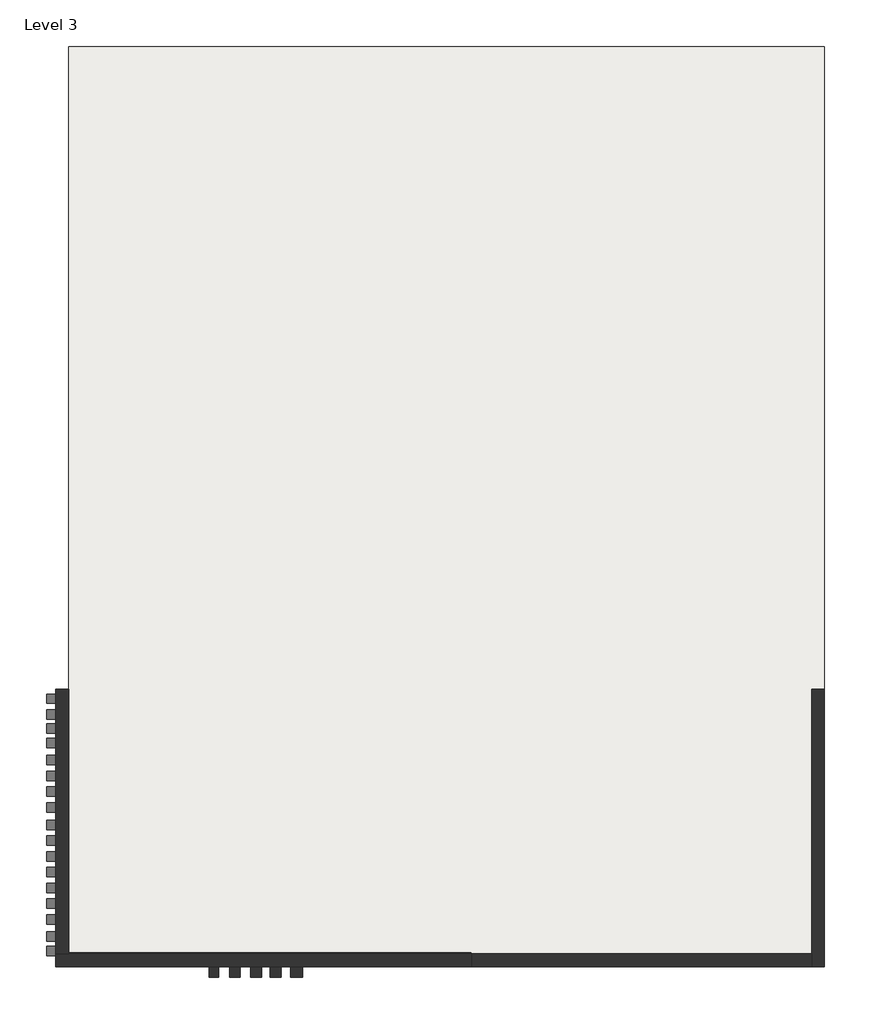
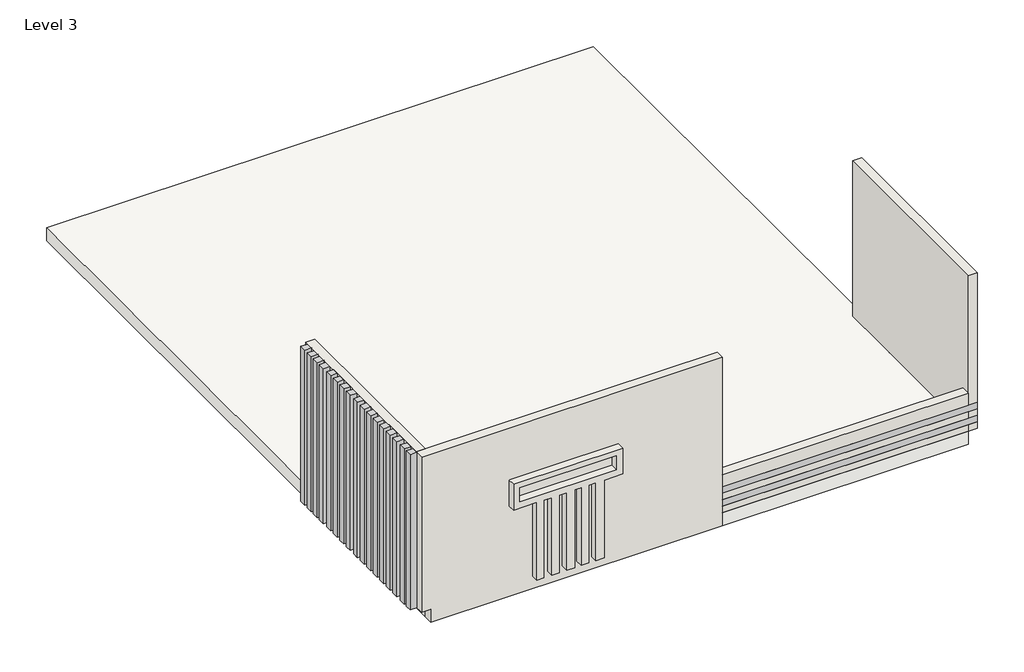
# One storey: 19 proxies, 5 walls, 1 roof.
"""IFC4 building model written with IfcOpenShell, lengths in millimetres."""

from ifc_helpers import new_model, si_unit, frame, origin, place, context, project, spatial, polyline, outline, extrude, faceted_brep, transform, mapped, element, save
from components import walls_8_walls_8_a9e6a938

model = new_model("IFC4")

# Units and contexts
model_context = context("Model", 3, world=origin())
ifc_project = project(units=[si_unit("LENGTHUNIT", "METRE", prefix="MILLI")], contexts=[model_context])

# Site, building, storey
site = spatial("IfcSite", under=ifc_project)
building = spatial("IfcBuilding", under=site)
storey = spatial("IfcBuildingStorey", under=building, Name="Level 3", Elevation=7315.2)

# Proxies
placement = place(None, origin())
element("IfcBuildingElementProxy", 1, Name="Cornice", ObjectType="Cornice", at=placement, inside=storey, context=model_context, shape_type="SweptSolid", body=[
    extrude(outline(polyline([(-8577.2311901, -3.9139512), (-8729.6311901, -3.9139512), (-8729.6311901, 148.4860488), (-8577.2311901, 148.4860488), (-8577.2311901, -3.9139512)])), frame((0.0, 0.0, 7620.0), z_axis=(0.0, 0.0, 1.0), x_axis=(1.0, 0.0, 0.0)), (0.0, 0.0, 1.0), 3657.6),
])
element("IfcBuildingElementProxy", 2, Name="Cornice", ObjectType="Cornice", at=placement, inside=storey, context=model_context, shape_type="SweptSolid", body=[
    extrude(outline(polyline([(-8577.2311901, -257.9139512), (-8729.6311901, -257.9139512), (-8729.6311901, -105.5139512), (-8577.2311901, -105.5139512), (-8577.2311901, -257.9139512)])), frame((0.0, 0.0, 7620.0), z_axis=(0.0, 0.0, 1.0), x_axis=(1.0, 0.0, 0.0)), (0.0, 0.0, 1.0), 3657.6),
])
element("IfcBuildingElementProxy", 3, Name="Cornice", ObjectType="Cornice", at=placement, inside=storey, context=model_context, shape_type="SweptSolid", body=[
    extrude(outline(polyline([(-8577.2311901, -486.5139512), (-8729.6311901, -486.5139512), (-8729.6311901, -334.1139512), (-8577.2311901, -334.1139512), (-8577.2311901, -486.5139512)])), frame((0.0, 0.0, 7620.0), z_axis=(0.0, 0.0, 1.0), x_axis=(1.0, 0.0, 0.0)), (0.0, 0.0, 1.0), 3657.6),
])
element("IfcBuildingElementProxy", 4, Name="Cornice", ObjectType="Cornice", at=placement, inside=storey, context=model_context, shape_type="SweptSolid", body=[
    extrude(outline(polyline([(-8577.2311901, -715.1139512), (-8729.6311901, -715.1139512), (-8729.6311901, -562.7139512), (-8577.2311901, -562.7139512), (-8577.2311901, -715.1139512)])), frame((0.0, 0.0, 7620.0), z_axis=(0.0, 0.0, 1.0), x_axis=(1.0, 0.0, 0.0)), (0.0, 0.0, 1.0), 3657.6),
])
element("IfcBuildingElementProxy", 5, Name="Cornice", ObjectType="Cornice", at=placement, inside=storey, context=model_context, shape_type="SweptSolid", body=[
    extrude(outline(polyline([(-8577.2311901, -994.5139512), (-8729.6311901, -994.5139512), (-8729.6311901, -842.1139512), (-8577.2311901, -842.1139512), (-8577.2311901, -994.5139512)])), frame((0.0, 0.0, 7620.0), z_axis=(0.0, 0.0, 1.0), x_axis=(1.0, 0.0, 0.0)), (0.0, 0.0, 1.0), 3657.6),
])
element("IfcBuildingElementProxy", 6, Name="Cornice", ObjectType="Cornice", at=placement, inside=storey, context=model_context, shape_type="SweptSolid", body=[
    extrude(outline(polyline([(-8577.2311901, -1248.5139512), (-8729.6311901, -1248.5139512), (-8729.6311901, -1096.1139512), (-8577.2311901, -1096.1139512), (-8577.2311901, -1248.5139512)])), frame((0.0, 0.0, 7620.0), z_axis=(0.0, 0.0, 1.0), x_axis=(1.0, 0.0, 0.0)), (0.0, 0.0, 1.0), 3657.6),
])
element("IfcBuildingElementProxy", 7, Name="Cornice", ObjectType="Cornice", at=placement, inside=storey, context=model_context, shape_type="SweptSolid", body=[
    extrude(outline(polyline([(-8577.2311901, -1502.5139512), (-8729.6311901, -1502.5139512), (-8729.6311901, -1350.1139512), (-8577.2311901, -1350.1139512), (-8577.2311901, -1502.5139512)])), frame((0.0, 0.0, 7620.0), z_axis=(0.0, 0.0, 1.0), x_axis=(1.0, 0.0, 0.0)), (0.0, 0.0, 1.0), 3657.6),
])
element("IfcBuildingElementProxy", 8, Name="Cornice", ObjectType="Cornice", at=placement, inside=storey, context=model_context, shape_type="SweptSolid", body=[
    extrude(outline(polyline([(-8577.2311901, -1756.5139512), (-8729.6311901, -1756.5139512), (-8729.6311901, -1604.1139512), (-8577.2311901, -1604.1139512), (-8577.2311901, -1756.5139512)])), frame((0.0, 0.0, 7620.0), z_axis=(0.0, 0.0, 1.0), x_axis=(1.0, 0.0, 0.0)), (0.0, 0.0, 1.0), 3657.6),
])
element("IfcBuildingElementProxy", 9, Name="Cornice", ObjectType="Cornice", at=placement, inside=storey, context=model_context, shape_type="SweptSolid", body=[
    extrude(outline(polyline([(-8577.2311901, -2035.9139512), (-8729.6311901, -2035.9139512), (-8729.6311901, -1883.5139512), (-8577.2311901, -1883.5139512), (-8577.2311901, -2035.9139512)])), frame((0.0, 0.0, 7620.0), z_axis=(0.0, 0.0, 1.0), x_axis=(1.0, 0.0, 0.0)), (0.0, 0.0, 1.0), 3657.6),
])
element("IfcBuildingElementProxy", 10, Name="Cornice", ObjectType="Cornice", at=placement, inside=storey, context=model_context, shape_type="SweptSolid", body=[
    extrude(outline(polyline([(-8577.2311901, -2289.9139512), (-8729.6311901, -2289.9139512), (-8729.6311901, -2137.5139512), (-8577.2311901, -2137.5139512), (-8577.2311901, -2289.9139512)])), frame((0.0, 0.0, 7620.0), z_axis=(0.0, 0.0, 1.0), x_axis=(1.0, 0.0, 0.0)), (0.0, 0.0, 1.0), 3657.6),
])
element("IfcBuildingElementProxy", 11, Name="Cornice", ObjectType="Cornice", at=placement, inside=storey, context=model_context, shape_type="SweptSolid", body=[
    extrude(outline(polyline([(-8577.2311901, -2543.9139512), (-8729.6311901, -2543.9139512), (-8729.6311901, -2391.5139512), (-8577.2311901, -2391.5139512), (-8577.2311901, -2543.9139512)])), frame((0.0, 0.0, 7620.0), z_axis=(0.0, 0.0, 1.0), x_axis=(1.0, 0.0, 0.0)), (0.0, 0.0, 1.0), 3657.6),
])
element("IfcBuildingElementProxy", 12, Name="Cornice", ObjectType="Cornice", at=placement, inside=storey, context=model_context, shape_type="SweptSolid", body=[
    extrude(outline(polyline([(-8577.2311901, -2797.9139512), (-8729.6311901, -2797.9139512), (-8729.6311901, -2645.5139512), (-8577.2311901, -2645.5139512), (-8577.2311901, -2797.9139512)])), frame((0.0, 0.0, 7620.0), z_axis=(0.0, 0.0, 1.0), x_axis=(1.0, 0.0, 0.0)), (0.0, 0.0, 1.0), 3657.6),
])
element("IfcBuildingElementProxy", 13, Name="Cornice", ObjectType="Cornice", at=placement, inside=storey, context=model_context, shape_type="SweptSolid", body=[
    extrude(outline(polyline([(-8577.2311901, -3051.9139512), (-8729.6311901, -3051.9139512), (-8729.6311901, -2899.5139512), (-8577.2311901, -2899.5139512), (-8577.2311901, -3051.9139512)])), frame((0.0, 0.0, 7620.0), z_axis=(0.0, 0.0, 1.0), x_axis=(1.0, 0.0, 0.0)), (0.0, 0.0, 1.0), 3657.6),
])
element("IfcBuildingElementProxy", 14, Name="Cornice", ObjectType="Cornice", at=placement, inside=storey, context=model_context, shape_type="SweptSolid", body=[
    extrude(outline(polyline([(-8577.2311901, -3305.9139512), (-8729.6311901, -3305.9139512), (-8729.6311901, -3153.5139512), (-8577.2311901, -3153.5139512), (-8577.2311901, -3305.9139512)])), frame((0.0, 0.0, 7620.0), z_axis=(0.0, 0.0, 1.0), x_axis=(1.0, 0.0, 0.0)), (0.0, 0.0, 1.0), 3657.6),
])
element("IfcBuildingElementProxy", 15, Name="Cornice", ObjectType="Cornice", at=placement, inside=storey, context=model_context, shape_type="SweptSolid", body=[
    extrude(outline(polyline([(-8577.2311901, -3559.9139512), (-8729.6311901, -3559.9139512), (-8729.6311901, -3407.5139512), (-8577.2311901, -3407.5139512), (-8577.2311901, -3559.9139512)])), frame((0.0, 0.0, 7620.0), z_axis=(0.0, 0.0, 1.0), x_axis=(1.0, 0.0, 0.0)), (0.0, 0.0, 1.0), 3657.6),
])
element("IfcBuildingElementProxy", 16, Name="Cornice", ObjectType="Cornice", at=placement, inside=storey, context=model_context, shape_type="SweptSolid", body=[
    extrude(outline(polyline([(-8577.2311901, -3839.3139512), (-8729.6311901, -3839.3139512), (-8729.6311901, -3686.9139512), (-8577.2311901, -3686.9139512), (-8577.2311901, -3839.3139512)])), frame((0.0, 0.0, 7620.0), z_axis=(0.0, 0.0, 1.0), x_axis=(1.0, 0.0, 0.0)), (0.0, 0.0, 1.0), 3657.6),
])
element("IfcBuildingElementProxy", 17, Name="Cornice", ObjectType="Cornice", at=placement, inside=storey, context=model_context, shape_type="SweptSolid", body=[
    extrude(outline(polyline([(-8577.2311901, -4067.9139512), (-8729.6311901, -4067.9139512), (-8729.6311901, -3915.5139512), (-8577.2311901, -3915.5139512), (-8577.2311901, -4067.9139512)])), frame((0.0, 0.0, 7620.0), z_axis=(0.0, 0.0, 1.0), x_axis=(1.0, 0.0, 0.0)), (0.0, 0.0, 1.0), 3657.6),
])
element("IfcBuildingElementProxy", 18, Name="Reveal", ObjectType="Reveal", at=placement, inside=storey, context=model_context, shape_type="SweptSolid", body=[
    extrude(outline(polyline([(-1871.6311901, -4245.7139512), (-1871.6311901, -4093.3139512), (3817.9688099, -4093.3139512), (3817.9688099, -4245.7139512), (-1871.6311901, -4245.7139512)])), frame((0.0, 0.0, 8077.2), z_axis=(0.0, 0.0, 1.0), x_axis=(1.0, 0.0, 0.0)), (0.0, 0.0, 1.0), 152.4),
])
element("IfcBuildingElementProxy", 19, Name="Reveal", ObjectType="Reveal", at=placement, inside=storey, context=model_context, shape_type="SweptSolid", body=[
    extrude(outline(polyline([(-1871.6311901, -4245.7139512), (-1871.6311901, -4093.3139512), (3817.9688099, -4093.3139512), (3817.9688099, -4245.7139512), (-1871.6311901, -4245.7139512)])), frame((0.0, 0.0, 7772.4), z_axis=(0.0, 0.0, 1.0), x_axis=(1.0, 0.0, 0.0)), (0.0, 0.0, 1.0), 152.4),
])

# Roof
element("IfcRoof", 20, ObjectType="Generic - 12\"", at=placement, inside=storey, context=model_context, shape_type="SweptSolid", body=[
    extrude(outline(polyline([(-8374.0311901, 10587.8860488), (3817.9688099, 10587.8860488), (3817.9688099, -1197.7139512), (3614.7688099, -1197.7139512), (3614.7688099, -4245.7139512), (-1871.6311901, -4245.7139512), (-1871.6311901, -4017.1139512), (-8374.0311901, -4017.1139512), (-8374.0311901, 10587.8860488)])), frame((0.0, 0.0, 7315.2), z_axis=(0.0, 0.0, 1.0), x_axis=(1.0, 0.0, 0.0)), (0.0, 0.0, 1.0), 304.8),
])

# Walls
element("IfcWall", 21, ObjectType="Generic - 8\"", at=placement, inside=storey, context=model_context, shape_type="Brep", body=[
    faceted_brep([(-1871.6311901, -4042.5139512, 11277.6), (-1871.6311901, -4042.5139512, 8515.7457285), (-1871.6311901, -4042.5139512, 7620.0), (-1871.6311901, -4042.5139512, 7315.2), (-8374.0311901, -4042.5139512, 7315.2), (-8374.0311901, -4042.5139512, 7620.0), (-8577.2311901, -4042.5139512, 7620.0), (-8577.2311901, -4042.5139512, 11277.6), (-8374.0311901, -4042.5139512, 11277.6), (-1871.6311901, -4245.7139512, 7315.2), (-1871.6311901, -4245.7139512, 7620.0), (-1871.6311901, -4245.7139512, 7772.4), (-1871.6311901, -4245.7139512, 7924.8), (-1871.6311901, -4245.7139512, 8077.2), (-1871.6311901, -4245.7139512, 8229.6), (-1871.6311901, -4245.7139512, 8515.7457285), (-1871.6311901, -4245.7139512, 11277.6), (-8577.2311901, -4245.7139512, 11277.6), (-8577.2311901, -4245.7139512, 7620.0), (-8374.0311901, -4245.7139512, 7620.0), (-8374.0311901, -4245.7139512, 7315.2)], [[[0, 1, 2, 3, 4, 5, 6, 7, 8]], [[9, 10, 11, 12, 13, 14, 15, 16, 17, 18, 19, 20]], [[4, 3, 9, 20]], [[0, 8, 7, 17, 16]], [[18, 6, 5, 19]], [[5, 4, 20, 19]], [[7, 6, 18, 17]], [[0, 16, 15, 14, 13, 12, 11, 10, 9, 3, 2, 1]]]),
])
element("IfcWall", 22, ObjectType="Generic - 8\"", at=placement, inside=storey, context=model_context, shape_type="Brep", body=[
    faceted_brep([(3817.9688099, -4245.7139512, 7620.0), (3817.9688099, 224.6860488, 7620.0), (3817.9688099, 224.6860488, 11277.6), (3817.9688099, -4245.7139512, 11277.6), (3817.9688099, -4245.7139512, 8229.6), (3817.9688099, -4093.3139512, 8229.6), (3817.9688099, -4093.3139512, 8077.2), (3817.9688099, -4245.7139512, 8077.2), (3817.9688099, -4245.7139512, 7924.8), (3817.9688099, -4093.3139512, 7924.8), (3817.9688099, -4093.3139512, 7772.4), (3817.9688099, -4245.7139512, 7772.4), (3614.7688099, 224.6860488, 7620.0), (3614.7688099, -4042.5139512, 7620.0), (3614.7688099, -4245.7139512, 7620.0), (3614.7688099, -4245.7139512, 7772.4), (3614.7688099, -4093.3139512, 7772.4), (3614.7688099, -4093.3139512, 7924.8), (3614.7688099, -4245.7139512, 7924.8), (3614.7688099, -4245.7139512, 8077.2), (3614.7688099, -4093.3139512, 8077.2), (3614.7688099, -4093.3139512, 8229.6), (3614.7688099, -4245.7139512, 8229.6), (3614.7688099, -4245.7139512, 8515.7457285), (3614.7688099, -4245.7139512, 11277.6), (3614.7688099, 224.6860488, 11277.6)], [[[0, 1, 2, 3, 4, 5, 6, 7, 8, 9, 10, 11]], [[12, 13, 14, 15, 16, 17, 18, 19, 20, 21, 22, 23, 24, 25]], [[1, 0, 14, 13, 12]], [[2, 1, 12, 25]], [[3, 2, 25, 24]], [[3, 24, 23, 22, 4]], [[14, 0, 11, 15]], [[7, 19, 18, 8]], [[21, 5, 4, 22]], [[5, 21, 20, 6]], [[6, 20, 19, 7]], [[17, 9, 8, 18]], [[9, 17, 16, 10]], [[10, 16, 15, 11]]]),
])
element("IfcWall", 23, ObjectType="Generic - 8\"", at=placement, inside=storey, context=model_context, shape_type="Brep", body=[
    faceted_brep([(-8374.0311901, -4042.5139512, 7620.0), (-8374.0311901, -1045.3139512, 7620.0), (-8374.0311901, 224.6860488, 7620.0), (-8374.0311901, 224.6860488, 11277.6), (-8374.0311901, -4042.5139512, 11277.6), (-8577.2311901, -4042.5139512, 7620.0), (-8577.2311901, -4042.5139512, 11277.6), (-8577.2311901, 224.6860488, 11277.6), (-8577.2311901, 224.6860488, 7620.0), (-8577.2311901, -1045.3139512, 7620.0)], [[[0, 1, 2, 3, 4]], [[5, 6, 7, 8, 9]], [[2, 1, 0, 5, 9, 8]], [[3, 2, 8, 7]], [[4, 3, 7, 6]], [[0, 4, 6, 5]]]),
])
element("IfcWall", 24, ObjectType="Generic - 8\"", at=placement, inside=storey, context=model_context, shape_type="SweptSolid", body=[
    extrude(outline(polyline([(-4042.5139512, 8515.7457285), (-4042.5139512, 7620.0), (-4245.7139512, 7620.0), (-4245.7139512, 7772.4), (-4093.3139512, 7772.4), (-4093.3139512, 7924.8), (-4245.7139512, 7924.8), (-4245.7139512, 8077.2), (-4093.3139512, 8077.2), (-4093.3139512, 8229.6), (-4245.7139512, 8229.6), (-4245.7139512, 8515.7457285), (-4042.5139512, 8515.7457285)])), frame((-1871.6311901, 0.0, 0.0), z_axis=(1.0, 0.0, 0.0), x_axis=(0.0, 1.0, 0.0)), (0.0, 0.0, 1.0), 5486.4),
])
walls_8_walls_8_shape = walls_8_walls_8_a9e6a938(model_context)
element("IfcWall", 25, ObjectType="Walls 8 : Walls 8", at=placement, inside=storey, context=model_context, shape_type="MappedRepresentation", body=[
    mapped(walls_8_walls_8_shape, transform((0.0, 0.0, 0.0), x_axis=(1.0, 0.0, 0.0), y_axis=(0.0, 1.0, 0.0), z_axis=(0.0, 0.0, 1.0))),
])

save(model, "model.ifc")

# Revit data of these elements
# Type "Generic - 12\""
#   Assembly Code = "B1020"
#   Layers, outside or top first: 1' - 0" no material (function 1)
# Type "Generic - 8\""
#   Assembly Code = "B2010"
#   Layers, outside or top first: 0' - 8" no material (function 1)
# Elements 1, 2, 3, 4, 5, 6, 7, 8, 9, 10, 11, 12, 13, 14, 15, 16, 17 (IfcBuildingElementProxy, "Cornice")
#   Phase Created = New Construction
#   Materials on its faces: "Default Wall"
# Element 20 (IfcRoof, "Generic - 12\"")
#   built-in parameter 1001705 = 25 (stored number, unit not read)
#   built-in parameter 1001710 = 33615
#   Phase Created = New Construction
#   Materials on its faces: "Default Roof"
# Element 21 (IfcWall, "Generic - 8\"")
#   Top Offset = 0' - 0"
#   Base Offset = 0' - 0"
#   Unconnected Height = 13' - 0"
#   wall height = 13' - 0"
#   Phase Created = New Construction
#   Base Constraint = Level 3
#   Materials on its faces: "Default Wall"
# Elements 22, 23 (IfcWall, "Generic - 8\"")
#   built-in parameter 1001111 = 1' - 0"
#   Top Offset = 0' - 0"
#   Base Offset = 1' - 0"
#   Unconnected Height = 12' - 0"
#   wall height = 12' - 0"
#   Phase Created = New Construction
#   Base Constraint = Level 3
#   Materials on its faces: "Default Wall"
# Element 24 (IfcWall, "Generic - 8\"")
#   built-in parameter 1001111 = 1' - 0"
#   Top Offset = 0' - 0"
#   Base Offset = 1' - 0"
#   Unconnected Height = 2' - 11.26558"
#   wall height = 2' - 11.26558"
#   Phase Created = New Construction
#   Base Constraint = Level 3
#   Materials on its faces: "Default Wall"
# Element 25 (IfcWall, "Walls 8 : Walls 8")
#   Phase Created = New Construction
#   Materials on its faces: "Default Wall"
# Materials
#   "Default Wall": colour RGB 128 128 128, transparency 0
#   "Default Roof": colour RGB 88 101 114, transparency 0
